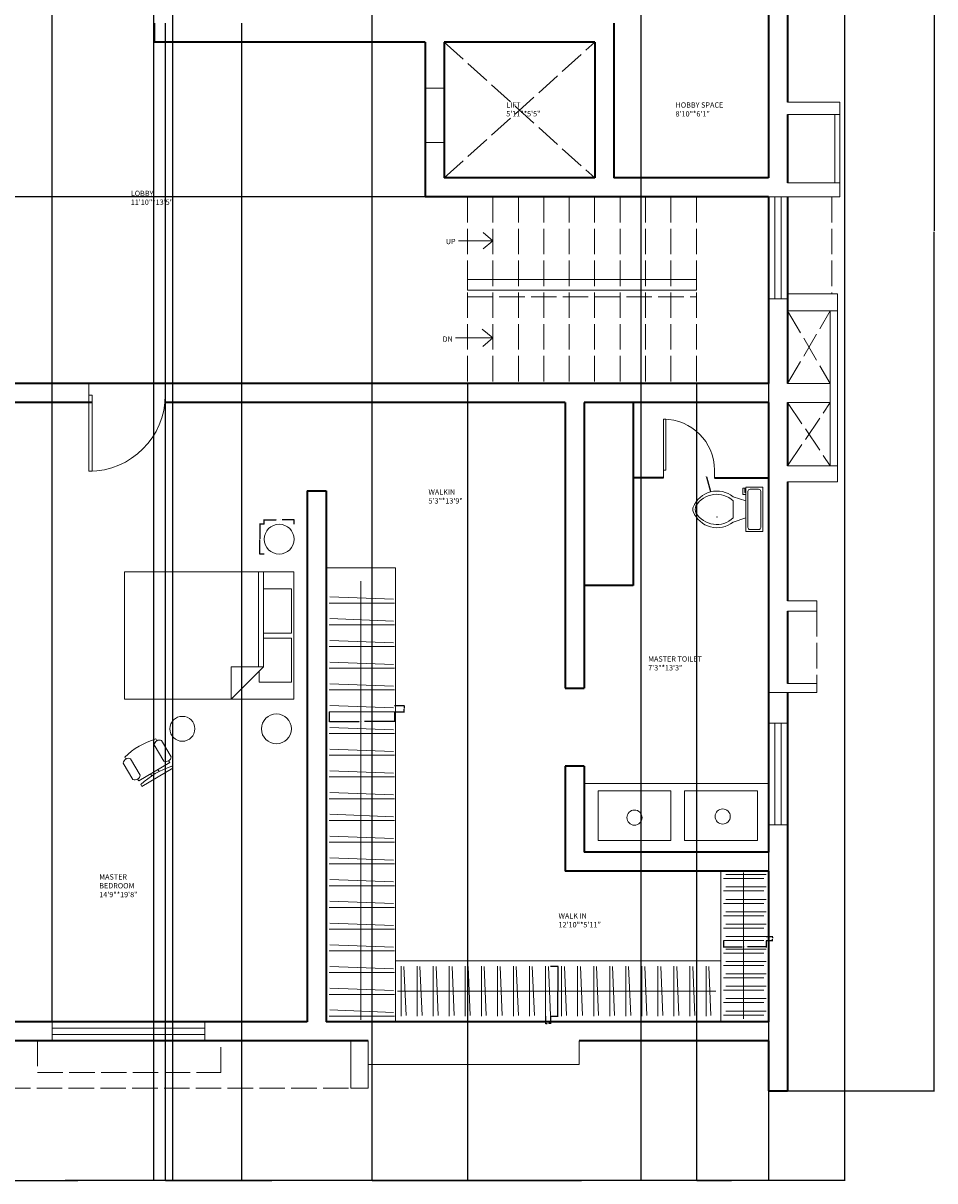
# Model space of a CAD drawing. Units: inches. Extents: x 293720 to 590083, y 155482 to 312405.
# Tile 2 of 4: x 294112 to 294542, y 155482 to 156028. Entities that reach past the tile are written whole.
import ezdxf

# ---------------------------------------------------------------- set-up
doc = ezdxf.new("R2010")
doc.units = ezdxf.units.IN
doc.linetypes.add('ACAD_ISO02W100', pattern=[15, 12, -3])
for name, color, linetype, lineweight in [('A-ANNO-DIMS', 2, 'Continuous', 18), ('A-ANNO-SYMB', 7, 'Continuous', 18), ('A-AREA-IDEN', 7, 'Continuous', 18), ('A-DOOR', 3, 'Continuous', 18), ('A-EQPM-ELEV', 4, 'Continuous', 18), ('A-FLOR-CASE', 8, 'Continuous', 18), ('A-FLOR-FIXT', 9, 'Continuous', 18), ('A-FLOR-OPEN', 8, 'ACAD_ISO02W100', 13), ('A-FLOR-OVHD', 8, 'ACAD_ISO02W100', 13), ('A-FLOR-PROJ', 8, 'Continuous', 18), ('A-FLOR-STRS', 7, 'Continuous', 18), ('A-FLOR-STRS-HIDN', 7, 'ACAD_ISO02W100', 18), ('A-FURN', 8, 'Continuous', 18), ('A-GLAZ', 4, 'Continuous', 18), ('A-WALL', 7, 'Continuous', 35)]:
    doc.layers.add(name, color=color, linetype=linetype, lineweight=lineweight)
doc.styles.get("Standard").update_dxf_attribs({"font": 'arial.ttf'})
doc.dimstyles.get("Standard").update_dxf_attribs({"dimtxt": 0.18, "dimasz": 0.18, "dimexe": 0.18, "dimexo": 0.0625, "dimgap": 0.09, "dimtad": 0, "dimtih": 1, "dimtoh": 1, "dimdec": 4, "dimzin": 0, "dimdsep": 46, "dimtxsty": 'Standard', "dimcen": 0.09, "dimadec": 0, "dimazin": 0, "dimtfac": 1, "dimtdec": 4, "dimtofl": 0, "dimtmove": 0, "dimatfit": 3, "dimfxl": 1, "dimtolj": 1, "dimtzin": 0, "dimarcsym": 0})

# ---------------------------------------------------------------- blocks, each defined once
blk = doc.blocks.new('Bed - Queen')
for p, q in [((0, -80.00003), (0, 0)), ((0, 0), (59.99999, 0)), ((59.99999, 0), (59.99999, -80.00003)), ((7.99999, -1.2), (28.79998, -1.2)), ((7.99999, -14.4), (7.99999, -1.2)), ((28.79998, -1.2), (28.79998, -14.4)), ((31.19999, -1.2), (51.99999, -1.2)), ((31.19999, -14.4), (31.19999, -1.2)), ((51.99999, -1.2), (51.99999, -16.4)), ((0, -14.4), (44.8, -14.4)), ((59.99999, -29.6), (44.8, -14.4)), ((44.8, -14.4), (44.8, -29.6)), ((44.8, -16.8), (0, -16.8)), ((51.99999, -16.4), (46.79936, -16.4)), ((44.8, -29.6), (59.99999, -29.6)), ((59.99999, -80.00003), (0, -80.00003))]:
    blk.add_line(p, q)
blk = doc.blocks.new('Toilet - top')
for p, q in [((9.5, -6), (9.5, -2)), ((-10, -8.5), (-8, -8.5)), ((-10, -9.5), (-10, -8.5)), ((-7, -9.5), (-10, -9.5)), ((-8, -8.5), (-8, -8)), ((-7, -8), (-7, -9.5)), ((-4, -8), (-6, -14)), ((4, -8), (6, -14)), ((4, -14), (-4, -14))]:
    blk.add_line(p, q)
blk.add_lwpolyline([(10.5, -8), (10.5, 0), (-10.5, 0), (-10.5, -8)], close=True)
for points in [[(-9.5, -2), (-9.5, -6)], [(8.5, -1), (-8.5, -1)], [(-8.5, -7), (8.5, -7)]]:
    blk.add_lwpolyline(points)
for centre, radius, start, end in [((-8.62, -1.88), 0.884, 81.8699, 188.1301), ((8.62, -1.88), 0.884, 351.8699, 98.1301), ((-8.62, -6.12), 0.884, 171.8699, 278.1301), ((8.62, -6.12), 0.884, 261.8699, 8.1301), ((3.52, -21.58), 12.17, 141.4691, 247.9714), ((4.2, -21.82), 11.33, 136.3677, 238.9468), ((-3.52, -21.58), 12.17, 292.0284, 38.5307), ((-4.2, -21.82), 11.33, 301.053, 43.6321), ((0, -27.88), 4, 245.7318, 294.2682), ((0, -29), 4, 254.8605, 285.1395)]:
    blk.add_arc(centre, radius, start, end)
blk = doc.blocks.new('Chair - Desk')
for p, q in [((-8.5, 0), (-8.5, -1)), ((-8.5, 0), (8.5, 0)), ((8.5, 0), (8.5, -1)), ((-10.5, -5), (-10.5, -14)), ((-8.5, -3), (-8.5, -4)), ((-8.5, -3), (8.5, -3)), ((-6.5, -14), (-6.5, -5)), ((-2, -3), (-2, -1.9355)), ((2, -1.9576), (2, -3)), ((6.5, -5), (6.5, -14)), ((8.5, -3), (8.5, -4)), ((10.5, -14), (10.5, -5)), ((-8.5, -15), (-8.5, -16)), ((8.5, -15), (8.5, -16))]:
    blk.add_line(p, q)
for centre, radius, start, end in [((-8.5, -6.5), 2.5, 36.8699, 143.1301), ((0, 34.625), 36.625, 256.5803, 283.4197), ((8.5, -6.5), 2.5, 36.8699, 143.1301), ((-8.5, -12.5), 2.5, 216.8699, 323.1301), ((0, 19.625), 36.625, 256.5803, 283.4197), ((8.5, -12.5), 2.5, 216.8699, 323.1301)]:
    blk.add_arc(centre, radius, start, end)
blk = doc.blocks.new('*U2')
for p, q in [((0, 0), (0, -6)), ((40, 0), (40, -6))]:
    blk.add_line(p, q)
blk.add_lwpolyline([(0, 0), (0, 40), (1.75, 40), (1.75, 0)], close=True)
blk.add_arc((0, 0), 40, 0, 90)
blk = doc.blocks.new('WIN-48IN')
for p, q in [((0, 9), (48, 9)), ((0, 0), (0, 9)), ((0, 6), (48, 6)), ((48, 9), (48, 0)), ((48, 3), (0, 3)), ((48, 0), (0, 0))]:
    blk.add_line(p, q)
blk = doc.blocks.new('WIN-72IN')
for p, q in [((0, 9), (72, 9)), ((0, 0), (0, 9)), ((0, 6), (72, 6)), ((72, 9), (72, 0)), ((72, 3), (0, 3)), ((72, 0), (0, 0))]:
    blk.add_line(p, q)
blk = doc.blocks.new('WARDROBE-HANGER-30P74IN')
for p, q in [((0, 0), (30.74, 0)), ((0.25, 2.89), (30.33, 1.77))]:
    blk.add_line(p, q)
blk = doc.blocks.new('WARDROBE-HANGER-23P51IN')
for p, q in [((0, 23.51), (0, 0)), ((1.34, 23.46), (2.32, 0.33))]:
    blk.add_line(p, q)
blk = doc.blocks.new('WARDROBE-HANGER-19P03IN')
for p, q in [((1.03, 1.89), (20.06, 1.89)), ((0, 0), (19.03, 0))]:
    blk.add_line(p, q)
blk = doc.blocks.new('NIGHTSTAND-ROUND')
blk.add_circle((7.05, 7.05), 7.05)
blk = doc.blocks.new('*D23')
at = {"layer": 'A-ANNO-DIMS', "color": 0, "lineweight": -2, "transparency": 16777216}
for p, q in [((294256.02, 155703.07), (294256.02, 155698.34)), ((294286.76, 155703.07), (294286.76, 155698.34)), ((294256.2, 155698.52), (294270.18, 155698.52)), ((294286.58, 155698.52), (294272.61, 155698.52))]:
    blk.add_line(p, q, dxfattribs=at)
at = {"layer": 'A-ANNO-DIMS', "color": 0, "lineweight": 100, "transparency": 16777216}
for points in [[(294256.2, 155698.55), (294256.2, 155698.49), (294256.02, 155698.52)], [(294286.58, 155698.55), (294286.58, 155698.49), (294286.76, 155698.52)]]:
    blk.add_solid(points, dxfattribs=at)
at = {"layer": 'Defpoints', "color": 0, "lineweight": 100, "transparency": 16777216}
for p in [(294256.02, 155703.13), (294286.76, 155703.13), (294286.76, 155698.52)]:
    blk.add_point(p, dxfattribs=at)
at = {"layer": 'A-ANNO-DIMS', "color": 0, "transparency": 16777216, "insert": (294271.39, 155698.52), "char_height": 0.18, "attachment_point": 5}
blk.add_mtext('\\A1;HANGER A 31 TYP.', dxfattribs=at)
blk = doc.blocks.new('*D24')
at = {"layer": 'A-ANNO-DIMS', "color": 0, "lineweight": -2, "transparency": 16777216}
for p, q in [((294286.83, 155706.01), (294291.56, 155706.01)), ((294286.83, 155703.13), (294291.56, 155703.13)), ((294291.38, 155705.83), (294291.38, 155704.75)), ((294291.38, 155703.31), (294291.38, 155704.39))]:
    blk.add_line(p, q, dxfattribs=at)
at = {"layer": 'A-ANNO-DIMS', "color": 0, "lineweight": 100, "transparency": 16777216}
for points in [[(294291.35, 155705.83), (294291.41, 155705.83), (294291.38, 155706.01)], [(294291.35, 155703.31), (294291.41, 155703.31), (294291.38, 155703.13)]]:
    blk.add_solid(points, dxfattribs=at)
at = {"layer": 'Defpoints', "color": 0, "lineweight": 100, "transparency": 16777216}
for p in [(294286.76, 155706.01), (294286.76, 155703.13), (294291.38, 155706.01)]:
    blk.add_point(p, dxfattribs=at)
at = {"layer": 'A-ANNO-DIMS', "color": 0, "transparency": 16777216, "insert": (294291.38, 155704.57), "char_height": 0.18, "attachment_point": 5}
blk.add_mtext('\\A1;3 TYP.', dxfattribs=at)
blk = doc.blocks.new('*D25')
at = {"layer": 'A-ANNO-DIMS', "color": 0, "lineweight": -2, "transparency": 16777216}
for p, q in [((294360.45, 155583.08), (294364.09, 155583.08)), ((294363.91, 155582.9), (294363.91, 155571.51)), ((294363.91, 155559.75), (294363.91, 155571.14)), ((294360.45, 155559.57), (294364.09, 155559.57))]:
    blk.add_line(p, q, dxfattribs=at)
at = {"layer": 'A-ANNO-DIMS', "color": 0, "lineweight": 100, "transparency": 16777216}
for points in [[(294363.88, 155582.9), (294363.94, 155582.9), (294363.91, 155583.08)], [(294363.88, 155559.75), (294363.94, 155559.75), (294363.91, 155559.57)]]:
    blk.add_solid(points, dxfattribs=at)
at = {"layer": 'Defpoints', "color": 0, "lineweight": 100, "transparency": 16777216}
for p in [(294360.38, 155583.08), (294363.91, 155583.08), (294360.38, 155559.57)]:
    blk.add_point(p, dxfattribs=at)
at = {"layer": 'A-ANNO-DIMS', "color": 0, "transparency": 16777216, "insert": (294363.91, 155571.33), "char_height": 0.18, "attachment_point": 5}
blk.add_mtext('\\A1;HANGER B 24 TYP.', dxfattribs=at)
blk = doc.blocks.new('*D26')
at = {"layer": 'A-ANNO-DIMS', "color": 0, "lineweight": -2, "transparency": 16777216}
for p, q in [((294358.06, 155559.51), (294358.06, 155555.87)), ((294358.24, 155556.05), (294358.77, 155556.05)), ((294360.2, 155556.05), (294359.68, 155556.05)), ((294360.38, 155559.51), (294360.38, 155555.87))]:
    blk.add_line(p, q, dxfattribs=at)
at = {"layer": 'A-ANNO-DIMS', "color": 0, "lineweight": 100, "transparency": 16777216}
for points in [[(294358.24, 155556.08), (294358.24, 155556.02), (294358.06, 155556.05)], [(294360.2, 155556.08), (294360.2, 155556.02), (294360.38, 155556.05)]]:
    blk.add_solid(points, dxfattribs=at)
at = {"layer": 'Defpoints', "color": 0, "lineweight": 100, "transparency": 16777216}
for p in [(294358.06, 155559.57), (294360.38, 155559.57), (294360.38, 155556.05)]:
    blk.add_point(p, dxfattribs=at)
at = {"layer": 'A-ANNO-DIMS', "color": 0, "transparency": 16777216, "insert": (294359.22, 155556.05), "char_height": 0.18, "attachment_point": 5}
blk.add_mtext('\\A1;2 TYP.', dxfattribs=at)
blk = doc.blocks.new('*D35')
at = {"layer": 'A-ANNO-DIMS', "color": 0, "lineweight": -2, "transparency": 16777216}
for p, q in [((294442.02, 155595.1), (294442.02, 155591.98)), ((294462.07, 155595.1), (294462.07, 155591.98)), ((294442.2, 155592.16), (294450.81, 155592.16)), ((294461.89, 155592.16), (294453.27, 155592.16))]:
    blk.add_line(p, q, dxfattribs=at)
at = {"layer": 'A-ANNO-DIMS', "color": 0, "lineweight": 100, "transparency": 16777216}
for points in [[(294442.2, 155592.19), (294442.2, 155592.13), (294442.02, 155592.16)], [(294461.89, 155592.19), (294461.89, 155592.13), (294462.07, 155592.16)]]:
    blk.add_solid(points, dxfattribs=at)
at = {"layer": 'Defpoints', "color": 0, "lineweight": 100, "transparency": 16777216}
for p in [(294442.02, 155595.17), (294462.07, 155595.17), (294462.07, 155592.16)]:
    blk.add_point(p, dxfattribs=at)
at = {"layer": 'A-ANNO-DIMS', "color": 0, "transparency": 16777216, "insert": (294452.04, 155592.16), "char_height": 0.18, "attachment_point": 5}
blk.add_mtext('\\A1;HANGER G 20 TYP.', dxfattribs=at)
blk = doc.blocks.new('*D36')
at = {"layer": 'A-ANNO-DIMS', "color": 0, "lineweight": -2, "transparency": 16777216}
for p, q in [((294462.13, 155597.05), (294465.26, 155597.05)), ((294462.13, 155595.17), (294465.26, 155595.17)), ((294465.08, 155596.87), (294465.08, 155596.29)), ((294465.08, 155595.35), (294465.08, 155595.93))]:
    blk.add_line(p, q, dxfattribs=at)
at = {"layer": 'A-ANNO-DIMS', "color": 0, "lineweight": 100, "transparency": 16777216}
for points in [[(294465.05, 155596.87), (294465.11, 155596.87), (294465.08, 155597.05)], [(294465.05, 155595.35), (294465.11, 155595.35), (294465.08, 155595.17)]]:
    blk.add_solid(points, dxfattribs=at)
at = {"layer": 'Defpoints', "color": 0, "lineweight": 100, "transparency": 16777216}
for p in [(294462.07, 155597.05), (294462.07, 155595.17), (294465.08, 155597.05)]:
    blk.add_point(p, dxfattribs=at)
at = {"layer": 'A-ANNO-DIMS', "color": 0, "transparency": 16777216, "insert": (294465.08, 155596.11), "char_height": 0.18, "attachment_point": 5}
blk.add_mtext('\\A1;2 TYP.', dxfattribs=at)
blk = doc.blocks.new('*D49')
at = {"layer": 'A-ANNO-DIMS', "color": 0, "lineweight": -2, "transparency": 16777216}
for p, q in [((294225.36, 155791.62), (294225.36, 155793.85)), ((294225.54, 155793.67), (294231.03, 155793.67)), ((294239.27, 155793.67), (294233.78, 155793.67)), ((294239.45, 155791.62), (294239.45, 155793.85))]:
    blk.add_line(p, q, dxfattribs=at)
at = {"layer": 'A-ANNO-DIMS', "color": 0, "lineweight": 100, "transparency": 16777216}
for points in [[(294225.54, 155793.7), (294225.54, 155793.64), (294225.36, 155793.67)], [(294239.27, 155793.7), (294239.27, 155793.64), (294239.45, 155793.67)]]:
    blk.add_solid(points, dxfattribs=at)
at = {"layer": 'Defpoints', "color": 0, "lineweight": 100, "transparency": 16777216}
for p in [(294225.36, 155791.56), (294239.45, 155793.67), (294239.45, 155791.56)]:
    blk.add_point(p, dxfattribs=at)
at = {"layer": 'A-ANNO-DIMS', "color": 0, "transparency": 16777216, "insert": (294232.4, 155793.67), "char_height": 0.18, "attachment_point": 5}
blk.add_mtext('\\A1;NIGHTSTAND 14 TYP.', dxfattribs=at)
blk = doc.blocks.new('*D50')
at = {"layer": 'A-ANNO-DIMS', "color": 0, "lineweight": -2, "transparency": 16777216}
for p, q in [((294225.3, 155791.56), (294223.06, 155791.56)), ((294223.24, 155791.38), (294223.24, 155784.69)), ((294223.24, 155777.64), (294223.24, 155784.33)), ((294225.3, 155777.46), (294223.06, 155777.46))]:
    blk.add_line(p, q, dxfattribs=at)
at = {"layer": 'A-ANNO-DIMS', "color": 0, "lineweight": 100, "transparency": 16777216}
for points in [[(294223.21, 155791.38), (294223.27, 155791.38), (294223.24, 155791.56)], [(294223.21, 155777.64), (294223.27, 155777.64), (294223.24, 155777.46)]]:
    blk.add_solid(points, dxfattribs=at)
at = {"layer": 'Defpoints', "color": 0, "lineweight": 100, "transparency": 16777216}
for p in [(294223.24, 155791.56), (294225.36, 155791.56), (294225.36, 155777.46)]:
    blk.add_point(p, dxfattribs=at)
at = {"layer": 'A-ANNO-DIMS', "color": 0, "transparency": 16777216, "insert": (294223.24, 155784.51), "char_height": 0.18, "attachment_point": 5}
blk.add_mtext('\\A1;14 TYP.', dxfattribs=at)
blk = doc.blocks.new('*D53')
at = {"layer": 'A-ANNO-DIMS', "color": 0, "lineweight": -2, "transparency": 16777216}
for p, q in [((294499.07, 156062.55), (294499.07, 155481.85)), ((293762.89, 155594.88), (293762.89, 155481.85)), ((293763.07, 155482.03), (294130.59, 155482.03)), ((294498.89, 155482.03), (294131.37, 155482.03))]:
    blk.add_line(p, q, dxfattribs=at)
at = {"layer": 'A-ANNO-DIMS', "color": 0, "lineweight": 100, "transparency": 16777216}
for points in [[(293763.07, 155482.06), (293763.07, 155482), (293762.89, 155482.03)], [(294498.89, 155482.06), (294498.89, 155482), (294499.07, 155482.03)]]:
    blk.add_solid(points, dxfattribs=at)
at = {"layer": 'Defpoints', "color": 0, "lineweight": 100, "transparency": 16777216}
for p in [(294499.07, 156062.61), (293762.89, 155594.94), (294499.07, 155482.03)]:
    blk.add_point(p, dxfattribs=at)
at = {"layer": 'A-ANNO-DIMS', "color": 0, "transparency": 16777216, "insert": (294130.98, 155482.03), "char_height": 0.18, "attachment_point": 5}
blk.add_mtext('\\A1;736.2', dxfattribs=at)
blk = doc.blocks.new('*D54')
at = {"layer": 'A-ANNO-DIMS', "color": 0, "lineweight": -2, "transparency": 16777216}
for p, q in [((294472.34, 156335.04), (294541.6, 156335.04)), ((294541.42, 156334.86), (294541.42, 155929.89)), ((294541.42, 155524.56), (294541.42, 155929.53)), ((294472.34, 155524.38), (294541.6, 155524.38))]:
    blk.add_line(p, q, dxfattribs=at)
at = {"layer": 'A-ANNO-DIMS', "color": 0, "lineweight": 100, "transparency": 16777216}
for points in [[(294541.39, 156334.86), (294541.45, 156334.86), (294541.42, 156335.04)], [(294541.39, 155524.56), (294541.45, 155524.56), (294541.42, 155524.38)]]:
    blk.add_solid(points, dxfattribs=at)
at = {"layer": 'Defpoints', "color": 0, "lineweight": 100, "transparency": 16777216}
for p in [(294472.28, 156335.04), (294541.42, 156335.04), (294472.28, 155524.38)]:
    blk.add_point(p, dxfattribs=at)
at = {"layer": 'A-ANNO-DIMS', "color": 0, "transparency": 16777216, "insert": (294541.42, 155929.71), "char_height": 0.18, "attachment_point": 5}
blk.add_mtext('\\A1;810.7', dxfattribs=at)
blk = doc.blocks.new('*D58')
at = {"layer": 'A-ANNO-DIMS', "color": 0, "lineweight": -2, "transparency": 16777216}
for p, q in [((294102.09, 156200.87), (294102.09, 155481.85)), ((294173.09, 156200.87), (294173.09, 155481.85)), ((294102.27, 155482.03), (294137.39, 155482.03)), ((294172.91, 155482.03), (294137.79, 155482.03))]:
    blk.add_line(p, q, dxfattribs=at)
at = {"layer": 'A-ANNO-DIMS', "color": 0, "lineweight": 100, "transparency": 16777216}
for points in [[(294102.27, 155482.06), (294102.27, 155482), (294102.09, 155482.03)], [(294172.91, 155482.06), (294172.91, 155482), (294173.09, 155482.03)]]:
    blk.add_solid(points, dxfattribs=at)
at = {"layer": 'Defpoints', "color": 0, "lineweight": 100, "transparency": 16777216}
for p in [(294102.09, 156200.93), (294173.09, 156200.93), (294173.09, 155482.03)]:
    blk.add_point(p, dxfattribs=at)
at = {"layer": 'A-ANNO-DIMS', "color": 0, "transparency": 16777216, "insert": (294137.59, 155482.03), "char_height": 0.18, "attachment_point": 5}
blk.add_mtext('\\A1;71', dxfattribs=at)
blk = doc.blocks.new('*D59')
at = {"layer": 'A-ANNO-DIMS', "color": 0, "lineweight": -2, "transparency": 16777216}
for p, q in [((294276.09, 156215.87), (294276.09, 155481.85)), ((294182.09, 156206.87), (294182.09, 155481.85)), ((294182.27, 155482.03), (294228.87, 155482.03)), ((294275.91, 155482.03), (294229.31, 155482.03))]:
    blk.add_line(p, q, dxfattribs=at)
at = {"layer": 'A-ANNO-DIMS', "color": 0, "lineweight": 100, "transparency": 16777216}
for points in [[(294182.27, 155482.06), (294182.27, 155482), (294182.09, 155482.03)], [(294275.91, 155482.06), (294275.91, 155482), (294276.09, 155482.03)]]:
    blk.add_solid(points, dxfattribs=at)
at = {"layer": 'Defpoints', "color": 0, "lineweight": 100, "transparency": 16777216}
for p in [(294276.09, 156215.93), (294182.09, 156206.93), (294276.09, 155482.03)]:
    blk.add_point(p, dxfattribs=at)
at = {"layer": 'A-ANNO-DIMS', "color": 0, "transparency": 16777216, "insert": (294229.09, 155482.03), "char_height": 0.18, "attachment_point": 5}
blk.add_mtext('\\A1;94', dxfattribs=at)
blk = doc.blocks.new('*D60')
at = {"layer": 'A-ANNO-DIMS', "color": 0, "lineweight": -2, "transparency": 16777216}
for p, q in [((294276.09, 156215.87), (294276.09, 155481.85)), ((294403.09, 156215.87), (294403.09, 155481.85)), ((294276.27, 155482.03), (294339.31, 155482.03)), ((294402.91, 155482.03), (294339.87, 155482.03))]:
    blk.add_line(p, q, dxfattribs=at)
at = {"layer": 'A-ANNO-DIMS', "color": 0, "lineweight": 100, "transparency": 16777216}
for points in [[(294276.27, 155482.06), (294276.27, 155482), (294276.09, 155482.03)], [(294402.91, 155482.06), (294402.91, 155482), (294403.09, 155482.03)]]:
    blk.add_solid(points, dxfattribs=at)
at = {"layer": 'Defpoints', "color": 0, "lineweight": 100, "transparency": 16777216}
for p in [(294276.09, 156215.93), (294403.09, 156215.93), (294403.09, 155482.03)]:
    blk.add_point(p, dxfattribs=at)
at = {"layer": 'A-ANNO-DIMS', "color": 0, "transparency": 16777216, "insert": (294339.59, 155482.03), "char_height": 0.18, "attachment_point": 5}
blk.add_mtext('\\A1;127', dxfattribs=at)
blk = doc.blocks.new('*D69')
at = {"layer": 'A-ANNO-DIMS', "color": 0, "lineweight": -2, "transparency": 16777216}
for p, q in [((294068.586085, 155556.990707), (294068.586085, 156377.567612)), ((294068.766085, 156377.387612), (294096.611145, 156377.387612)), ((294125.103763, 156377.387612), (294097.258703, 156377.387612)), ((294125.283763, 155556.990707), (294125.283763, 156377.567612))]:
    blk.add_line(p, q, dxfattribs=at)
at = {"layer": 'A-ANNO-DIMS', "color": 0, "lineweight": 100, "transparency": 16777216}
for points in [[(294068.766085, 156377.417612), (294068.766085, 156377.357612), (294068.586085, 156377.387612)], [(294125.103763, 156377.417612), (294125.103763, 156377.357612), (294125.283763, 156377.387612)]]:
    blk.add_solid(points, dxfattribs=at)
at = {"layer": 'Defpoints', "color": 0, "lineweight": 100, "transparency": 16777216}
for p in [(294125.283763, 156377.387612), (294068.586085, 155556.928207), (294125.283763, 155556.928207)]:
    blk.add_point(p, dxfattribs=at)
at = {"layer": 'A-ANNO-DIMS', "color": 0, "transparency": 16777216, "insert": (294096.934924, 156377.387612), "char_height": 0.18, "attachment_point": 5}
blk.add_mtext('\\A1;56.7', dxfattribs=at)
blk = doc.blocks.new('*D70')
at = {"layer": 'A-ANNO-DIMS', "color": 0, "lineweight": -2, "transparency": 16777216}
for p, q in [((294321.24, 155857.87), (294321.24, 155481.85)), ((294429.24, 155857.87), (294429.24, 155481.85)), ((294321.42, 155482.03), (294374.96, 155482.03)), ((294429.06, 155482.03), (294375.52, 155482.03))]:
    blk.add_line(p, q, dxfattribs=at)
at = {"layer": 'A-ANNO-DIMS', "color": 0, "lineweight": 100, "transparency": 16777216}
for points in [[(294321.42, 155482.06), (294321.42, 155482), (294321.24, 155482.03)], [(294429.06, 155482.06), (294429.06, 155482), (294429.24, 155482.03)]]:
    blk.add_solid(points, dxfattribs=at)
at = {"layer": 'Defpoints', "color": 0, "lineweight": 100, "transparency": 16777216}
for p in [(294321.24, 155857.93), (294429.24, 155857.93), (294429.24, 155482.03)]:
    blk.add_point(p, dxfattribs=at)
at = {"layer": 'A-ANNO-DIMS', "color": 0, "transparency": 16777216, "insert": (294375.24, 155482.03), "char_height": 0.18, "attachment_point": 5}
blk.add_mtext('\\A1;108', dxfattribs=at)
blk = doc.blocks.new('*D71')
at = {"layer": 'A-ANNO-DIMS', "color": 0, "lineweight": -2, "transparency": 16777216}
for p, q in [((294429.24, 155857.87), (294429.24, 155481.85)), ((294463.28, 155857.87), (294463.28, 155481.85)), ((294429.42, 155482.03), (294445.86, 155482.03)), ((294463.1, 155482.03), (294446.65, 155482.03))]:
    blk.add_line(p, q, dxfattribs=at)
at = {"layer": 'A-ANNO-DIMS', "color": 0, "lineweight": 100, "transparency": 16777216}
for points in [[(294429.42, 155482.06), (294429.42, 155482), (294429.24, 155482.03)], [(294463.1, 155482.06), (294463.1, 155482), (294463.28, 155482.03)]]:
    blk.add_solid(points, dxfattribs=at)
at = {"layer": 'Defpoints', "color": 0, "lineweight": 100, "transparency": 16777216}
for p in [(294429.24, 155857.93), (294463.28, 155857.93), (294463.28, 155482.03)]:
    blk.add_point(p, dxfattribs=at)
at = {"layer": 'A-ANNO-DIMS', "color": 0, "transparency": 16777216, "insert": (294446.26, 155482.03), "char_height": 0.18, "attachment_point": 5}
blk.add_mtext('\\A1;34.04', dxfattribs=at)
blk = doc.blocks.new('*D72')
at = {"layer": 'A-ANNO-DIMS', "color": 0, "lineweight": -2, "transparency": 16777216}
for p, q in [((294321.18, 155945.93), (293720.36, 155945.93)), ((293720.54, 155945.75), (293720.54, 155902.11)), ((293720.54, 155858.11), (293720.54, 155901.75)), ((294321.18, 155857.93), (293720.36, 155857.93))]:
    blk.add_line(p, q, dxfattribs=at)
at = {"layer": 'A-ANNO-DIMS', "color": 0, "lineweight": 100, "transparency": 16777216}
for points in [[(293720.51, 155945.75), (293720.57, 155945.75), (293720.54, 155945.93)], [(293720.51, 155858.11), (293720.57, 155858.11), (293720.54, 155857.93)]]:
    blk.add_solid(points, dxfattribs=at)
at = {"layer": 'Defpoints', "color": 0, "lineweight": 100, "transparency": 16777216}
for p in [(293720.54, 155945.93), (294321.24, 155945.93), (294321.24, 155857.93)]:
    blk.add_point(p, dxfattribs=at)
at = {"layer": 'A-ANNO-DIMS', "color": 0, "transparency": 16777216, "insert": (293720.54, 155901.93), "char_height": 0.18, "attachment_point": 5}
blk.add_mtext('\\A1;88', dxfattribs=at)
blk = doc.blocks.new('*D73')
at = {"layer": 'A-ANNO-DIMS', "color": 0, "lineweight": -2, "transparency": 16777216}
for p, q in [((294178.56, 156027.87), (294178.56, 155481.85)), ((294214.56, 156027.87), (294214.56, 155481.85)), ((294178.74, 155482.03), (294196.34, 155482.03)), ((294214.38, 155482.03), (294196.77, 155482.03))]:
    blk.add_line(p, q, dxfattribs=at)
at = {"layer": 'A-ANNO-DIMS', "color": 0, "lineweight": 100, "transparency": 16777216}
for points in [[(294178.74, 155482.06), (294178.74, 155482), (294178.56, 155482.03)], [(294214.38, 155482.06), (294214.38, 155482), (294214.56, 155482.03)]]:
    blk.add_solid(points, dxfattribs=at)
at = {"layer": 'Defpoints', "color": 0, "lineweight": 100, "transparency": 16777216}
for p in [(294178.56, 156027.93), (294214.56, 156027.93), (294214.56, 155482.03)]:
    blk.add_point(p, dxfattribs=at)
at = {"layer": 'A-ANNO-DIMS', "color": 0, "transparency": 16777216, "insert": (294196.56, 155482.03), "char_height": 0.18, "attachment_point": 5}
blk.add_mtext('\\A1;36', dxfattribs=at)
blk = doc.blocks.new('*D81')
at = {"layer": 'A-ANNO-DIMS', "color": 0, "lineweight": -2, "transparency": 16777216}
for p, q in [((294433.86, 155813.88), (294434.04, 155813.88)), ((294434.04, 155813.88), (294435.85, 155806.99)), ((294438.9, 155795.05), (294439.08, 155795.05)), ((294438.99, 155794.96), (294438.99, 155795.14))]:
    blk.add_line(p, q, dxfattribs=at)
at = {"layer": 'A-ANNO-DIMS', "color": 0, "lineweight": 100, "transparency": 16777216}
blk.add_solid([(294435.88, 155807), (294435.82, 155806.99), (294435.89, 155806.82)], dxfattribs=at)
at = {"layer": 'Defpoints', "color": 0, "lineweight": 100, "transparency": 16777216}
for p in [(294435.89, 155806.82), (294438.99, 155795.05)]:
    blk.add_point(p, dxfattribs=at)
at = {"layer": 'A-ANNO-DIMS', "color": 0, "transparency": 16777216, "insert": (294433.18, 155813.88), "char_height": 0.18, "attachment_point": 5}
blk.add_mtext('\\A1;6X R12.17', dxfattribs=at)

msp = doc.modelspace()

# ---------------------------------------------------------------- linework, layer by layer
at = {"layer": 'A-ANNO-SYMB'}
for p, q in [((294333.239, 155925.304), (294328.6754, 155929.1145)), ((294317.0151, 155925.304), (294333.239, 155925.304)), ((294333.239, 155925.304), (294328.6754, 155921.4055)), ((294333.239, 155879.4301), (294328.1959, 155883.6465)), ((294315.6653, 155879.4301), (294333.239, 155879.4301)), ((294333.239, 155879.4301), (294328.4666, 155875.4451))]:
    msp.add_line(p, q, dxfattribs=at)
at = {"layer": 'A-EQPM-ELEV'}
for p, q in [((294301.2763, 155997.2808), (294310.2763, 155997.2808)), ((294301.2763, 155971.6338), (294310.2763, 155971.6338))]:
    msp.add_line(p, q, dxfattribs=at)
at = {"layer": 'A-FLOR-CASE'}
for p, q in [((294254.5861, 155771.0377), (294287.2585, 155771.0377)), ((294287.2585, 155771.0377), (294287.2585, 155556.9282)), ((294270.8746, 155557.8563), (294270.8746, 155764.7309)), ((294376.2763, 155669.2083), (294463.2763, 155669.2083)), ((294440.688, 155585.603), (294440.688, 155627.9282)), ((294451.5302, 155558.2409), (294451.5302, 155627.3145)), ((294287.2585, 155585.603), (294440.688, 155585.603)), ((294440.688, 155585.603), (294440.688, 155556.9282)), ((294288.2722, 155571.3265), (294438.4222, 155571.3265))]:
    msp.add_line(p, q, dxfattribs=at)
at = {"layer": 'A-FLOR-FIXT'}
for points in [[(294382.8268, 155665.8591), (294417.1622, 155665.8591), (294417.1622, 155642.315), (294382.8268, 155642.315)], [(294423.6707, 155665.8591), (294458.0061, 155665.8591), (294458.0061, 155642.315), (294423.6707, 155642.315)]]:
    msp.add_lwpolyline(points, close=True, dxfattribs=at)
for centre in [(294400.0079, 155653.1809), (294441.6377, 155653.7416)]:
    msp.add_circle(centre, 3.5793, dxfattribs=at)
at = {"layer": 'A-FLOR-OPEN'}
for p, q in [((294310.2763, 156018.9282), (294381.2763, 155954.9282)), ((294310.2763, 155954.9282), (294381.2763, 156018.9282)), ((294472.2763, 155892.2413), (294492.3713, 155857.9282)), ((294472.2763, 155857.9282), (294492.3713, 155892.2413)), ((294472.2763, 155848.9282), (294492.3713, 155819.1707)), ((294472.2763, 155819.1707), (294492.3713, 155848.9282))]:
    msp.add_line(p, q, dxfattribs=at)
at = {"layer": 'A-FLOR-OVHD'}
for p, q in [((294493.1325, 155945.9282), (294493.1325, 155900.2903)), ((294486.0949, 155750.5767), (294486.0949, 155716.4913)), ((294118.3918, 155547.9282), (294118.3918, 155532.9552)), ((294204.9419, 155532.9552), (294204.9419, 155547.9282)), ((294118.3918, 155532.9552), (294204.9419, 155532.9552)), ((293803.0931, 155525.5662), (294266.2589, 155525.5662))]:
    msp.add_line(p, q, dxfattribs=at)
at = {"layer": 'A-FLOR-PROJ'}
for p, q in [((294496.8318, 155990.6883), (294472.2763, 155990.6883)), ((294496.8318, 155984.8106), (294496.8318, 155990.6883)), ((294472.2763, 155984.8106), (294496.8318, 155984.8106)), ((294494.5904, 155984.8106), (294494.5904, 155952.5506)), ((294496.8318, 155984.8106), (294496.8318, 155952.5506)), ((294496.8318, 155952.5506), (294472.2763, 155952.5506)), ((294496.8318, 155945.9282), (294496.8318, 155952.5506)), ((294463.2763, 155945.9282), (294496.8318, 155945.9282)), ((294495.736, 155900.2903), (294472.2763, 155900.2903)), ((294495.736, 155892.2413), (294495.736, 155900.2903)), ((294472.2763, 155892.2413), (294495.736, 155892.2413)), ((294492.3713, 155892.2413), (294492.3713, 155819.1707)), ((294495.736, 155892.2413), (294495.736, 155819.1707)), ((294472.2763, 155857.9282), (294492.3713, 155857.9282)), ((294495.736, 155857.9282), (294495.736, 155848.9282)), ((294492.3713, 155848.9282), (294472.2763, 155848.9282)), ((294472.2763, 155819.1707), (294495.736, 155819.1707)), ((294495.736, 155819.1707), (294495.736, 155811.615)), ((294495.736, 155811.615), (294472.2763, 155811.615)), ((294472.2763, 155755.4753), (294486.0949, 155755.4753)), ((294486.0949, 155755.4753), (294486.0949, 155750.5767)), ((294486.0949, 155750.5767), (294472.2763, 155750.5767)), ((294472.2763, 155716.4913), (294486.0949, 155716.4913)), ((294486.0949, 155716.4913), (294486.0949, 155712.1779)), ((294486.0949, 155712.1779), (294463.2763, 155712.1779)), ((294266.2589, 155525.5662), (294266.2589, 155547.9282)), ((294274.4362, 155525.5662), (294274.4362, 155547.9282)), ((294373.854, 155536.7472), (294373.854, 155547.9282)), ((294274.4362, 155536.7472), (294373.854, 155536.7472)), ((294266.2589, 155525.5662), (294274.4362, 155525.5662))]:
    msp.add_line(p, q, dxfattribs=at)
at = {"layer": 'A-FLOR-STRS'}
for p, q in [((294429.239, 155907.0747), (294321.239, 155907.0747)), ((294321.239, 155907.0747), (294321.239, 155901.9282)), ((294429.239, 155901.9282), (294429.239, 155907.0747)), ((294321.239, 155901.9282), (294429.239, 155901.9282))]:
    msp.add_line(p, q, dxfattribs=at)
at = {"layer": 'A-FLOR-STRS-HIDN'}
for p, q in [((294321.239, 155945.9282), (294321.239, 155857.9282)), ((294333.239, 155945.9282), (294333.239, 155857.9282)), ((294345.239, 155945.9282), (294345.239, 155857.9282)), ((294357.239, 155945.9282), (294357.239, 155857.9282)), ((294369.239, 155945.9282), (294369.239, 155857.9282)), ((294381.239, 155945.9282), (294381.239, 155857.9282)), ((294393.239, 155945.9282), (294393.239, 155857.9282)), ((294405.239, 155945.9282), (294405.239, 155857.9282)), ((294417.239, 155945.9282), (294417.239, 155857.9282)), ((294429.239, 155945.9282), (294429.239, 155857.9282)), ((294321.239, 155898.8673), (294429.239, 155898.8673))]:
    msp.add_line(p, q, dxfattribs=at)
at = {"layer": 'A-FURN'}
msp.add_circle((294186.7681, 155695.0747), 5.8857, dxfattribs=at)
at = {"layer": 'A-WALL'}
for p, q in [((294472.2763, 156313.9282), (294472.2763, 155990.6883)), ((294463.2763, 156304.9282), (294463.2763, 155954.9282)), ((294173.4975, 156027.9282), (294173.4975, 156018.9282)), ((294390.2763, 156027.9282), (294390.2763, 155954.9282)), ((294301.2763, 156018.9282), (294173.4975, 156018.9282)), ((294301.2763, 156018.9282), (294301.2763, 155945.9282)), ((294310.2763, 156018.9282), (294310.2763, 155954.9282)), ((294381.2763, 156018.9282), (294310.2763, 156018.9282)), ((294381.2763, 156018.9282), (294381.2763, 155954.9282)), ((294472.2763, 155984.8106), (294472.2763, 155952.5506)), ((294381.2763, 155954.9282), (294310.2763, 155954.9282)), ((294463.2763, 155954.9282), (294390.2763, 155954.9282)), ((294463.2763, 155945.9282), (294301.2763, 155945.9282)), ((294463.2763, 155945.9282), (294463.2763, 155857.9282)), ((294472.2763, 155945.9282), (294472.2763, 155857.9282)), ((294463.2763, 155857.9282), (294025.2305, 155857.9282)), ((294144.2603, 155848.9282), (294025.2305, 155848.9282)), ((294367.2763, 155848.9282), (294178.5048, 155848.9282)), ((294367.2763, 155848.9282), (294367.2763, 155714.2768)), ((294463.2763, 155848.9282), (294376.2763, 155848.9282)), ((294376.2763, 155848.9282), (294376.2763, 155714.2768)), ((294399.406, 155848.9282), (294399.406, 155762.7239)), ((294463.2763, 155848.9282), (294463.2763, 155636.9282)), ((294472.2763, 155848.9282), (294472.2763, 155819.1707)), ((294413.7326, 155813.5119), (294399.406, 155813.5119)), ((294437.7326, 155813.5119), (294463.2763, 155813.5119)), ((294472.2763, 155811.615), (294472.2763, 155755.4753)), ((294245.5861, 155807.4019), (294245.5861, 155556.9282)), ((294245.5861, 155807.4019), (294254.5861, 155807.4019)), ((294254.5861, 155807.4019), (294254.5861, 155556.9282)), ((294399.406, 155762.7239), (294376.2763, 155762.7239)), ((294472.2763, 155750.5767), (294472.2763, 155716.4913)), ((294367.2763, 155714.2768), (294376.2763, 155714.2768)), ((294472.2763, 155712.1779), (294472.2763, 155524.3834)), ((294376.2763, 155677.5088), (294367.2763, 155677.5088)), ((294367.2763, 155677.5088), (294367.2763, 155627.9282)), ((294376.2763, 155677.5088), (294376.2763, 155636.9282)), ((294463.2763, 155636.9282), (294376.2763, 155636.9282)), ((294463.2763, 155627.9282), (294367.2763, 155627.9282)), ((294463.2763, 155627.9282), (294463.2763, 155556.9282)), ((294245.5861, 155556.9282), (294068.5861, 155556.9282)), ((294463.2763, 155556.9282), (294254.5861, 155556.9282)), ((294274.4362, 155547.9282), (293803.0931, 155547.9282)), ((294463.2763, 155547.9282), (294373.854, 155547.9282)), ((294463.2763, 155547.9282), (294463.2763, 155524.3834)), ((294463.2763, 155524.3834), (294472.2763, 155524.3834))]:
    msp.add_line(p, q, dxfattribs=at)

# ---------------------------------------------------------------- block references
at = {"layer": 'A-DOOR', "xscale": -0.9, "yscale": 0.9, "zscale": 0.9, "rotation": 180}
msp.add_blockref('*U2', (294142.6853, 155852.5282), dxfattribs=at)
at = {"layer": 'A-DOOR', "xscale": 0.6, "yscale": 0.6, "zscale": 0.6}
msp.add_blockref('*U2', (294413.7326, 155817.1119), dxfattribs=at)
at = {"layer": 'A-FLOR-CASE'}
for name, p in [('WARDROBE-HANGER-30P74IN', (294256.02, 155754.4029)), ('WARDROBE-HANGER-30P74IN', (294256.02, 155744.1478)), ('WARDROBE-HANGER-30P74IN', (294256.02, 155733.8927)), ('WARDROBE-HANGER-30P74IN', (294256.02, 155723.6376)), ('WARDROBE-HANGER-30P74IN', (294256.02, 155713.3825)), ('WARDROBE-HANGER-30P74IN', (294256.02, 155703.1274)), ('WARDROBE-HANGER-30P74IN', (294256.02, 155692.8723)), ('WARDROBE-HANGER-30P74IN', (294256.02, 155682.6172)), ('WARDROBE-HANGER-30P74IN', (294256.02, 155672.3621)), ('WARDROBE-HANGER-30P74IN', (294256.02, 155662.107)), ('WARDROBE-HANGER-30P74IN', (294256.02, 155651.8519)), ('WARDROBE-HANGER-30P74IN', (294256.02, 155641.5968)), ('WARDROBE-HANGER-30P74IN', (294256.02, 155631.3417)), ('WARDROBE-HANGER-19P03IN', (294442.015, 155624.4314)), ('WARDROBE-HANGER-30P74IN', (294256.02, 155621.0866)), ('WARDROBE-HANGER-19P03IN', (294442.015, 155618.5782)), ('WARDROBE-HANGER-30P74IN', (294256.02, 155610.8315)), ('WARDROBE-HANGER-19P03IN', (294442.015, 155612.7251)), ('WARDROBE-HANGER-19P03IN', (294442.015, 155606.872)), ('WARDROBE-HANGER-30P74IN', (294256.02, 155600.5764)), ('WARDROBE-HANGER-19P03IN', (294442.015, 155601.0189)), ('WARDROBE-HANGER-30P74IN', (294256.02, 155590.3213)), ('WARDROBE-HANGER-19P03IN', (294442.015, 155595.1657)), ('WARDROBE-HANGER-19P03IN', (294442.015, 155589.3126)), ('WARDROBE-HANGER-30P74IN', (294256.02, 155580.0662)), ('WARDROBE-HANGER-23P51IN', (294289.916, 155559.573)), ('WARDROBE-HANGER-23P51IN', (294297.4881, 155559.573)), ('WARDROBE-HANGER-23P51IN', (294305.0602, 155559.573)), ('WARDROBE-HANGER-23P51IN', (294312.6324, 155559.573)), ('WARDROBE-HANGER-23P51IN', (294320.2045, 155559.573)), ('WARDROBE-HANGER-23P51IN', (294327.7766, 155559.573)), ('WARDROBE-HANGER-23P51IN', (294335.3487, 155559.573)), ('WARDROBE-HANGER-23P51IN', (294342.9209, 155559.573)), ('WARDROBE-HANGER-23P51IN', (294350.493, 155559.573)), ('WARDROBE-HANGER-23P51IN', (294358.0651, 155559.573)), ('WARDROBE-HANGER-23P51IN', (294365.6372, 155559.573)), ('WARDROBE-HANGER-23P51IN', (294373.2094, 155559.573)), ('WARDROBE-HANGER-23P51IN', (294380.7815, 155559.573)), ('WARDROBE-HANGER-23P51IN', (294388.3536, 155559.573)), ('WARDROBE-HANGER-23P51IN', (294395.9257, 155559.573)), ('WARDROBE-HANGER-23P51IN', (294403.4979, 155559.573)), ('WARDROBE-HANGER-23P51IN', (294411.07, 155559.573)), ('WARDROBE-HANGER-23P51IN', (294418.6421, 155559.573)), ('WARDROBE-HANGER-23P51IN', (294426.2142, 155559.573)), ('WARDROBE-HANGER-23P51IN', (294433.7864, 155559.573)), ('WARDROBE-HANGER-19P03IN', (294442.015, 155583.4595)), ('WARDROBE-HANGER-19P03IN', (294442.015, 155577.6064)), ('WARDROBE-HANGER-30P74IN', (294256.02, 155569.8111)), ('WARDROBE-HANGER-19P03IN', (294442.015, 155571.7532)), ('WARDROBE-HANGER-19P03IN', (294442.015, 155565.9001)), ('WARDROBE-HANGER-30P74IN', (294256.02, 155559.556)), ('WARDROBE-HANGER-19P03IN', (294442.015, 155560.047))]:
    msp.add_blockref(name, p, dxfattribs=at)
at = {"layer": 'A-FLOR-FIXT', "rotation": 270}
msp.add_blockref('Toilet - top', (294460.5658, 155798.5702), dxfattribs=at)
at = {"layer": 'A-FURN'}
for p in [(294225.3574, 155777.4647), (294224.049, 155687.996)]:
    msp.add_blockref('NIGHTSTAND-ROUND', p, dxfattribs=at)
for name, p, rotation in [('Bed - Queen', (294239.3872, 155769.0671), 270), ('Chair - Desk', (294174.9738, 155672.2145), 210.5245848146129)]:
    msp.add_blockref(name, p, dxfattribs=dict(at, rotation=rotation))
at = {"layer": 'A-GLAZ', "rotation": 90.00000000013426}
for p in [(294472.2765, 155897.9285), (294472.2765, 155649.7207)]:
    msp.add_blockref('WIN-48IN', p, dxfattribs=at)
at = {"layer": 'A-GLAZ'}
msp.add_blockref('WIN-72IN', (294125.284, 155547.928), dxfattribs=at)

# ---------------------------------------------------------------- texts
at = {"layer": 'A-ANNO-SYMB', "char_height": 2.5, "attachment_point": 1}
for s, width, insert in [('UP', 10.280942, (294311.0255, 155926.1837)), ('DN', 12.394781, (294309.5104, 155880.1509))]:
    msp.add_mtext_dynamic_manual_height_columns(s, width=width, gutter_width=12.5, heights=[0], dxfattribs=dict(at, insert=insert))
at = {"layer": 'A-AREA-IDEN', "char_height": 2.5, "attachment_point": 1}
for s, width, insert in [('LIFT\\P5\'11"*5\'5"', 32.608362, (294339.5189, 155990.6111)), ('HOBBY SPACE\\P8\'10"*6\'1"', 45.514972, (294419.393, 155990.5659)), ('LOBBY\\P11\'10"*13\'5"', 130.255139, (294162.4055, 155948.8793)), ('WALKIN\\P5\'3"*13\'9"', 63.865087, (294302.8473, 155807.9961)), ('MASTER TOILET\\P7\'3"*13\'3"', 55.418047, (294406.4726, 155729.2713)), ('MASTER\\PBEDROOM\\P14\'9"*19\'8"', 88.103091, (294147.5153, 155626.4642)), ('WALK IN\\P12\'10"*5\'11"', 89.308755, (294364.1995, 155608.0671))]:
    msp.add_mtext_dynamic_manual_height_columns(s, width=width, gutter_width=12.5, heights=[0], dxfattribs=dict(at, insert=insert))

# ---------------------------------------------------------------- dimensions: what is measured, and where the dimension line sits
at = {"layer": 'A-ANNO-DIMS'}
for base, p1, p2, override, picture, middle in [((294125.2838, 156377.3876), (294068.5861, 155556.9282), (294125.2838, 155556.9282), {"dimdec": 1, "dimlfac": 1, "dimrnd": 0, "dimzin": 0, "dimdsep": 46, "dimlunit": 2}, '*D69', (294096.9349, 156377.3876)), ((294276.0931, 155482.0334), (294182.0931, 156206.9282), (294276.0931, 156215.9282), {"dimdec": 0, "dimlfac": 1, "dimrnd": 0, "dimzin": 0, "dimdsep": 46, "dimlunit": 2}, '*D59', (294229.0931, 155482.0334)), ((294403.0931, 155482.0334), (294276.0931, 156215.9282), (294403.0931, 156215.9282), {"dimdec": 0, "dimlfac": 1, "dimrnd": 0, "dimzin": 0, "dimdsep": 46, "dimlunit": 2}, '*D60', (294339.5931, 155482.0334)), ((294173.0931, 155482.0334), (294102.0931, 156200.9282), (294173.0931, 156200.9282), {"dimdec": 0, "dimlfac": 1, "dimrnd": 0, "dimzin": 0, "dimdsep": 46, "dimlunit": 2}, '*D58', (294137.5931, 155482.0334)), ((294499.0676, 155482.0334), (293762.8891, 155594.9386), (294499.0676, 156062.6102), {"dimdec": 1, "dimlfac": 1, "dimrnd": 0, "dimzin": 0, "dimdsep": 46, "dimlunit": 2}, '*D53', (294130.9783, 155482.0334)), ((294214.5558, 155482.0334), (294178.5558, 156027.9282), (294214.5558, 156027.9282), {"dimdec": 0, "dimlfac": 1, "dimrnd": 0, "dimzin": 0, "dimdsep": 46, "dimlunit": 2}, '*D73', (294196.5558, 155482.0334)), ((294429.239, 155482.0334), (294321.239, 155857.9282), (294429.239, 155857.9282), {"dimdec": 0, "dimlfac": 1, "dimrnd": 0, "dimzin": 0, "dimdsep": 46, "dimlunit": 2}, '*D70', (294375.239, 155482.0334)), ((294463.2763, 155482.0334), (294429.239, 155857.9282), (294463.2763, 155857.9282), {"dimdec": 2, "dimlfac": 1, "dimrnd": 0, "dimzin": 0, "dimdsep": 46, "dimlunit": 2}, '*D71', (294446.2577, 155482.0334))]:
    dim = msp.add_linear_dim(base=base, p1=p1, p2=p2, dimstyle='Standard', override=override, dxfattribs=at)
    dim.commit()
    dim.dimension.update_dxf_attribs({"geometry": picture, "text_midpoint": middle})
for base, p1, p2, override, picture, middle in [((294541.4176, 156335.0376), (294472.2763, 155524.3834), (294472.2763, 156335.0376), {"dimdec": 1, "dimlfac": 1, "dimrnd": 0, "dimzin": 0, "dimdsep": 46, "dimlunit": 2}, '*D54', (294541.4176, 155929.7105)), ((293720.5391, 155945.9282), (294321.239, 155857.9282), (294321.239, 155945.9282), {"dimdec": 0, "dimlfac": 1, "dimrnd": 0, "dimzin": 0, "dimdsep": 46, "dimlunit": 2}, '*D72', (293720.5391, 155901.9282))]:
    dim = msp.add_linear_dim(base=base, p1=p1, p2=p2, angle=90, dimstyle='Standard', override=override, dxfattribs=at)
    dim.commit()
    dim.dimension.update_dxf_attribs({"geometry": picture, "text_midpoint": middle})
dim = msp.add_radius_dim(center=(294438.9853, 155795.0506), mpoint=(294435.893, 155806.8202), text='6X <>', dimstyle='Standard', override={"dimdec": 2, "dimlfac": 1, "dimrnd": 0, "dimzin": 0, "dimdsep": 46, "dimlunit": 2}, dxfattribs=at)
dim.commit()
dim.dimension.update_dxf_attribs({"geometry": '*D81', "text_midpoint": (294433.1839, 155813.8819), "dimtype": 164})
for base, p1, p2, text, picture, middle in [((294223.2438, 155791.5564), (294225.3576, 155777.4646), (294225.3576, 155791.5564), '<> TYP.', '*D50', (294223.2438, 155784.5105)), ((294291.3762, 155706.0129), (294286.7644, 155703.1278), (294286.7644, 155706.0129), '<> TYP.', '*D24', (294291.3762, 155704.5703)), ((294465.0788, 155597.0542), (294462.0705, 155595.1654), (294462.0705, 155597.0542), '<> TYP.', '*D36', (294465.0788, 155596.1098)), ((294363.9107, 155583.0795), (294360.3848, 155559.5734), (294360.3848, 155583.0795), 'HANGER B <> TYP.', '*D25', (294363.9107, 155571.3265))]:
    dim = msp.add_linear_dim(base=base, p1=p1, p2=p2, angle=90, text=text, dimstyle='Standard', override={"dimdec": 0, "dimlfac": 1, "dimrnd": 0, "dimzin": 0, "dimdsep": 46, "dimlunit": 2}, dxfattribs=at)
    dim.commit()
    dim.dimension.update_dxf_attribs({"geometry": picture, "text_midpoint": middle})
for base, p1, p2, text, picture, middle in [((294239.4493, 155793.6701), (294225.3576, 155791.5564), (294239.4493, 155791.5564), 'NIGHTSTAND <> TYP.', '*D49', (294232.4035, 155793.6701)), ((294286.7644, 155698.5161), (294256.0195, 155703.1278), (294286.7644, 155703.1278), 'HANGER A <> TYP.', '*D23', (294271.392, 155698.5161)), ((294462.0705, 155592.1571), (294442.0152, 155595.1654), (294462.0705, 155595.1654), 'HANGER G <> TYP.', '*D35', (294452.0428, 155592.1571)), ((294360.3848, 155556.0475), (294358.0649, 155559.5734), (294360.3848, 155559.5734), '<> TYP.', '*D26', (294359.2248, 155556.0475))]:
    dim = msp.add_linear_dim(base=base, p1=p1, p2=p2, text=text, dimstyle='Standard', override={"dimdec": 0, "dimlfac": 1, "dimrnd": 0, "dimzin": 0, "dimdsep": 46, "dimlunit": 2}, dxfattribs=at)
    dim.commit()
    dim.dimension.update_dxf_attribs({"geometry": picture, "text_midpoint": middle})

doc.saveas('drawing.dxf')
